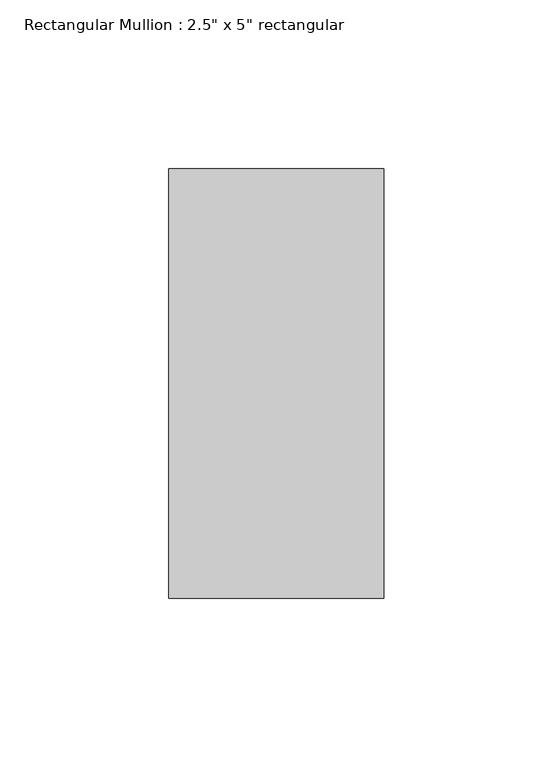
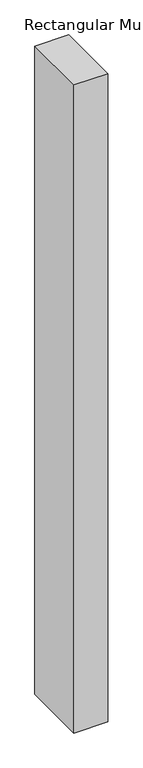
"""IFC4 building model written with IfcOpenShell, lengths in millimetres: member geometry."""

from ifc_helpers import new_model, si_unit, frame, origin, place, context, project, spatial, polyline, outline, extrude, source, transform, mapped, element, save


def member_093c7ff9(model_context):
    return source(origin(), model_context, "Body", "SweptSolid", [
        extrude(outline(polyline([(0.0, 63.5), (0.0, -63.5), (-63.5, -63.5), (-63.5, 63.5), (0.0, 63.5)])), frame((0.0, 0.0, -1288.9615505), z_axis=(0.0, 0.0, 1.0), x_axis=(1.0, 0.0, 0.0)), (0.0, 0.0, 1.0), 1288.9615505),
    ])


if __name__ == "__main__":
    model = new_model("IFC4")
    model_context = context("Model", 3, world=origin())
    ifc_project = project(units=[si_unit("LENGTHUNIT", "METRE", prefix="MILLI")], contexts=[model_context])
    site = spatial("IfcSite", under=ifc_project)
    building = spatial("IfcBuilding", under=site)
    placement = place(None, origin())
    member_shape = member_093c7ff9(model_context)
    element("IfcMember", 1, ObjectType="Rectangular Mullion : 2.5\" x 5\" rectangular", at=placement, inside=building, context=model_context, shape_type="MappedRepresentation", body=[
        mapped(member_shape, transform((0.0, 0.0, 0.0), x_axis=(1.0, 0.0, 0.0), y_axis=(0.0, 1.0, 0.0), z_axis=(0.0, 0.0, 1.0))),
    ])
    save(model, "model.ifc")

# Revit data of these elements
# Type "Rectangular Mullion : 2.5\" x 5\" rectangular"
#   built-in parameter 1007304 = 0.416667 (stored number, unit not read)
#   built-in parameter 1007301 = 0.104167 (stored number, unit not read)
#   built-in parameter 1007300 = 0.104167 (stored number, unit not read)
# Element 1 (IfcMember, "Rectangular Mullion : 2.5\" x 5\" rectangular")
#   Materials on its faces: "Aluminum"
# Materials
#   "Aluminum": class "Metal", colour RGB 247 247 247, transparency 0, Description = "Aluminum 6061", Cost = 0
